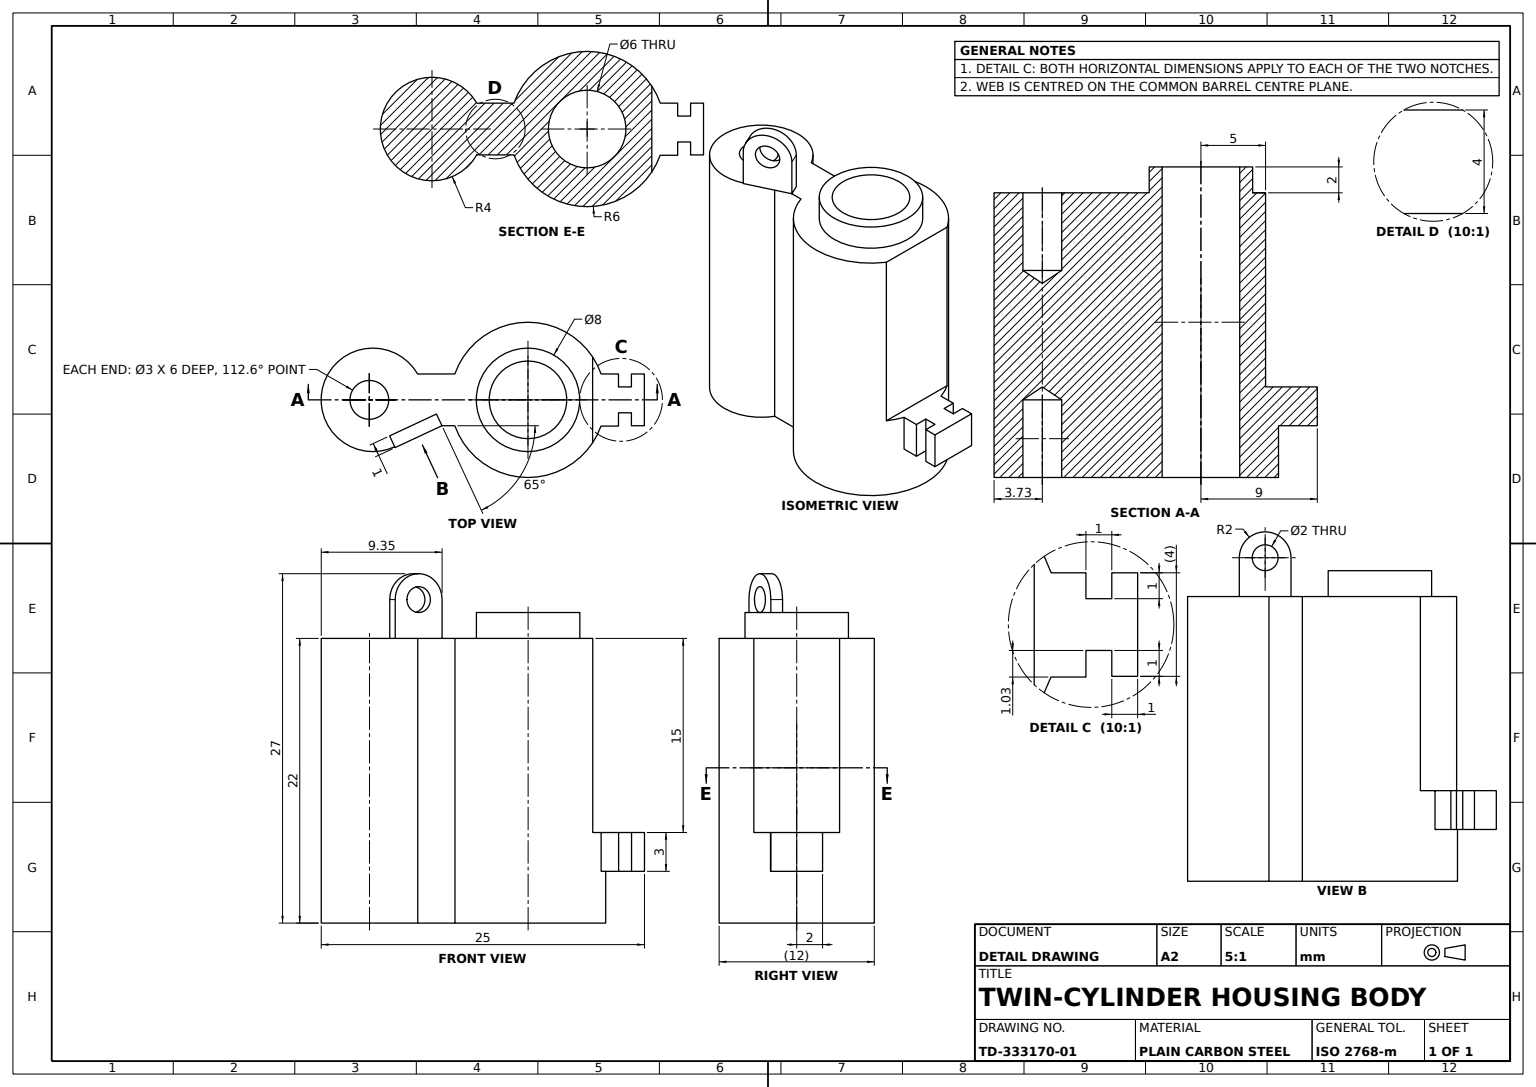
from build123d import *
from build123d.topology import SkipClean

# Parameters (mm, degrees)
TWIN_BARREL_BODY_DEPTH = 22
EYE_TAB_DEPTH          = 3
EYE_TAB_BOSS_DEPTH     = 1
EYE_HOLE_SKETCH_R      = 1
EYE_HOLE_2_DEPTH       = 1
COLLAR_RING_SKETCH_R   = 4
COLLAR_RING_SKETCH_R_2 = 3
COLLAR_RING_8_DEPTH    = 2
COLLAR_BORE_SKETCH_R   = 3
COLLAR_BORE_CUT_DEPTH  = 28.856776554
NOTCHED_START          = -3
NOTCHED_LUG_DEPTH      = 3
LUG_SLOT_CUT_DEPTH     = 27.305892876


with BuildPart() as part:
    # Twin Barrel Profile Sketch → Twin Barrel Body (new body)
    with BuildSketch(Plane(origin=(0, 0, 0), x_dir=(1, 0, 0), z_dir=(0, 1, 0))):
        with BuildLine():
            Line((-8.535898385, 2), (-5.656854249, 2))
            ThreePointArc((-5.656854249, 2), (6, 0), (-5.656854249, -2))
            Line((-5.656854249, -2), (-8.535898385, -2))
            ThreePointArc((-8.535898385, -2), (-16, 0), (-8.535898385, 2))
        make_face()
    extrude(amount=TWIN_BARREL_BODY_DEPTH)

    # Eye Tab Sketch → Eye Tab (add)
    with BuildSketch(Plane(origin=(0, 22, 0), x_dir=(1, 0, 0), z_dir=(0, 1, 0))):
        Polygon((-10.701722418, -2.78416526), (-8.889106844, -1.938928736), (-7.07649127, -1.093692213), (-6.653873008, -2), (-10.279104156, -3.690473047), align=None)
    extrude(amount=EYE_TAB_DEPTH)

    # Eye Tab Boss Sketch → Eye Tab Boss (add)
    with BuildSketch(Plane(origin=(-0.422378498, 0, -0.905793612), x_dir=(0.9063077870366508, 0, -0.4226182617406976), z_dir=(0.4226182617406976, 0, 0.9063077870366508))):
        with BuildLine():
            Line((-10.875693444, 25), (-6.875693444, 25))
            ThreePointArc((-6.875693444, 25), (-8.875693444, 27), (-10.875693444, 25))
        make_face()
    extrude(amount=-EYE_TAB_BOSS_DEPTH)

    # Eye Hole Sketch → Eye Hole Ø2 (cut)
    with BuildSketch(Plane(origin=(-0.422378498, 0, -0.905793612), x_dir=(0.9063077870366508, 0, -0.4226182617406976), z_dir=(0.4226182617406976, 0, 0.9063077870366508))):
        with Locations((-8.875693444, 25)):
            Circle(EYE_HOLE_SKETCH_R)
    extrude(amount=-EYE_HOLE_2_DEPTH, mode=Mode.SUBTRACT)

    # Barrel Bore Profile Sketch → Barrel Bore Cut (revolve, cut)
    with BuildSketch(Plane.XY, mode=Mode.PRIVATE) as barrel_bore_cut_sk:
        Polygon((-12.267949192, 22), (-12.267949192, 15), (-13.767949192, 16), (-13.767949192, 22), align=None)
    barrel_bore_cut = revolve(barrel_bore_cut_sk.sketch.rotate(Axis((-12.267949192, 22, 0), (0, -1, 0)), 270), axis=Axis((-12.267949192, 22, 0), (0, -1, 0)), mode=Mode.SUBTRACT)

    # Barrel Bore Mirror: Barrel Bore Cut across plane
    add(barrel_bore_cut.mirror(Plane.ZX.offset(11)), mode=Mode.SUBTRACT)

    # Collar Ring Sketch → Collar Ring Ø8 (add)
    with BuildSketch(Plane(origin=(0, 22, 0), x_dir=(1, 0, 0), z_dir=(0, 1, 0))):
        with Locations(Location((0, 0, 0), (0, 0, 270))):
            Circle(COLLAR_RING_SKETCH_R)
        with Locations(Location((0, 0, 0), (0, 0, 270))):
            Circle(COLLAR_RING_SKETCH_R_2, mode=Mode.SUBTRACT)
    extrude(amount=COLLAR_RING_8_DEPTH)

    # Collar Bore Sketch → Collar Bore Cut (cut, through all)
    with BuildSketch(Plane(origin=(0, 22, 0), x_dir=(1, 0, 0), z_dir=(0, 1, 0))):
        with Locations(Location((0, 0, 0), (0, 0, 270))):
            Circle(COLLAR_BORE_SKETCH_R)
    extrude(amount=-COLLAR_BORE_CUT_DEPTH, mode=Mode.SUBTRACT)

    # Notched Lug Sketch → Notched Lug (add)
    with SkipClean():  # the faces are left unmerged after this step: merging them gives an invalid solid
        with BuildSketch(Plane(origin=(0, 7, 0), x_dir=(1, 0, 0), z_dir=(0, 1, 0)).offset(NOTCHED_START)):
            with BuildLine():
                Line((5, 3.31662479), (5, -3.31662479))
                ThreePointArc((5, -3.31662479), (5.362357836, -2.691675768), (5.646981669, -2.027707579))
                Line((5.646981669, -2.027707579), (7, -2.027707579))
                Line((7, -2.027707579), (7, -1))
                Line((7, -1), (8, -1))
                Line((8, -1), (8, -2))
                Line((8, -2), (9, -2))
                Line((9, -2), (9, 2))
                Line((9, 2), (8, 2))
                Line((8, 2), (8, 1))
                Line((8, 1), (7, 1))
                Line((7, 1), (7, 2))
                Line((7, 2), (5.656854249, 2))
                ThreePointArc((5.656854249, 2), (5.368939451, 2.678523692), (5, 3.31662479))
            make_face()
        extrude(amount=NOTCHED_LUG_DEPTH)

    # Lug Slot Sketch → Lug Slot Cut (cut, through all)
    with SkipClean():  # the faces are left unmerged after this step: merging them gives an invalid solid
        with BuildSketch(Plane(origin=(0, 7, 0), x_dir=(1, 0, 0), z_dir=(0, 1, 0))):
            with BuildLine():
                Line((5, 3.31662479), (5, -3.31662479))
                ThreePointArc((5, -3.31662479), (5.362357836, -2.691675768), (5.646981669, -2.027707579))
                ThreePointArc((5.646981669, -2.027707579), (5.956511293, 0.721091683), (5, 3.31662479))
            make_face()
        extrude(amount=LUG_SLOT_CUT_DEPTH, mode=Mode.SUBTRACT)


solid = part.part
